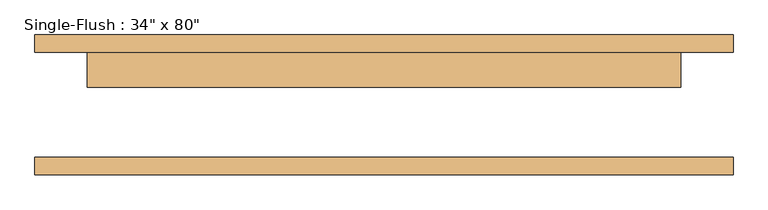
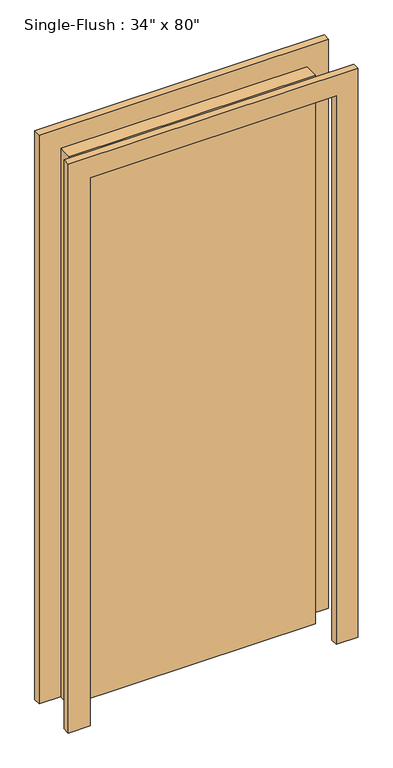
"""IFC4 building model written with IfcOpenShell, lengths in millimetres: door geometry."""

from ifc_helpers import new_model, si_unit, frame, origin, origin_with_axes, place, context, project, spatial, polyline, outline, extrude, source, transform, mapped, element, save


def door_56e8e0a9(model_context):
    return source(origin(), model_context, "Body", "SweptSolid", [
        extrude(outline(polyline([(2108.2, -508.0), (0.0, -508.0), (0.0, -431.8), (2032.0, -431.8), (2032.0, 431.8), (0.0, 431.8), (0.0, 508.0), (2108.2, 508.0), (2108.2, -508.0)])), frame((0.0, 76.2, 0.0), z_axis=(0.0, 1.0, 0.0), x_axis=(0.0, 0.0, 1.0)), (0.0, 0.0, 1.0), 25.4),
        extrude(outline(polyline([(2108.2, 508.0), (2108.2, -508.0), (0.0, -508.0), (0.0, -431.8), (2032.0, -431.8), (2032.0, 431.8), (0.0, 431.8), (0.0, 508.0), (2108.2, 508.0)])), frame((0.0, -101.6, 0.0), z_axis=(0.0, 1.0, 0.0), x_axis=(0.0, 0.0, 1.0)), (0.0, 0.0, 1.0), 25.4),
        extrude(outline(polyline([(431.8, 25.4), (-431.8, 25.4), (-431.8, 76.2), (431.8, 76.2), (431.8, 25.4)])), origin_with_axes(), (0.0, 0.0, 1.0), 2032.0),
    ])


if __name__ == "__main__":
    model = new_model("IFC4")
    model_context = context("Model", 3, world=origin())
    ifc_project = project(units=[si_unit("LENGTHUNIT", "METRE", prefix="MILLI")], contexts=[model_context])
    site = spatial("IfcSite", under=ifc_project)
    building = spatial("IfcBuilding", under=site)
    placement = place(None, origin())
    door_shape = door_56e8e0a9(model_context)
    element("IfcDoor", 1, ObjectType="Single-Flush : 34\" x 80\"", at=placement, inside=building, context=model_context, shape_type="MappedRepresentation", body=[
        mapped(door_shape, transform((0.0, 0.0, 0.0), x_axis=(1.0, 0.0, 0.0), y_axis=(0.0, 1.0, 0.0), z_axis=(0.0, 0.0, 1.0))),
    ])
    save(model, "model.ifc")

# Revit data of these elements
# Type "Single-Flush : 34\" x 80\""
#   Type Mark = "7"
#   Construction Type Id = "MDOOR"
#   Assembly Code = "C1020"
#   Analytic Construction = "Metal"
#   Thickness = 0' - 2"
#   Heat Transfer Coefficient (U) = 0.651978 BTU/(h·ft²·°F)
#   Height = 6' - 8"
#   Trim Projection Ext = 0' - 1"
#   Trim Projection Int = 0' - 1"
#   Trim Width = 0' - 3"
#   Width = 2' - 10"
#   Define Thermal Properties by = 1
#   Define Thermal Properties by = 1
#   Door Material = Door - Panel
#   Frame Material = Door - Frame
#   Visual Light Transmittance = 0
#   Solar Heat Gain Coefficient = 0
#   Function = (empty or 0)
#   Wall Closure = (empty or 0)
# Element 1 (IfcDoor, "Single-Flush : 34\" x 80\"")
#   Materials on its faces: "Door - Frame", "Door - Panel"
# Materials
#   "Door - Panel": class "Wood", colour RGB 210 159 95, transparency 0, Cost = 0
#   "Door - Frame": colour RGB 118 70 51, transparency 0, Cost = 0
